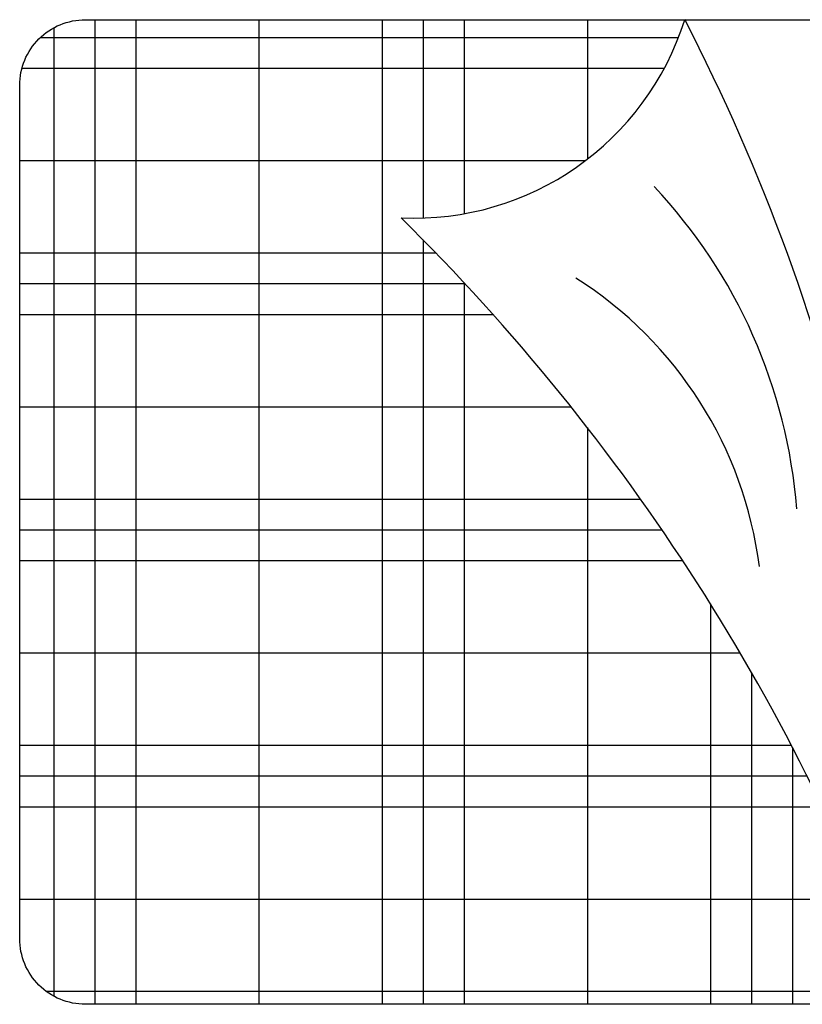
# Model space of a CAD drawing. Units: inches. Extents: x 3064 to 19385, y 846 to 15425.
# Tile 68 of 108: x 6533 to 6580, y 1625 to 1685. Entities that reach past the tile are written whole.
import ezdxf

# ---------------------------------------------------------------- set-up
doc = ezdxf.new("R2010")
doc.units = ezdxf.units.IN
doc.layers.add('A-FLOR-FIXT', color=9, linetype='Continuous', lineweight=18)
doc.layers.add('BLOCK', color=6, linetype='Continuous')

# ---------------------------------------------------------------- blocks, each defined once
blk = doc.blocks.new('*X5')
at = {"color": 0}
for p, q in [((276.598, 451.25), (280.51, 451.25)), ((275.455, 450.625), (280.51, 450.625)), ((274.411, 450), (280.51, 450)), ((265.51, 448.125), (267.634, 448.125)), ((271.723, 448.125), (280.51, 448.125)), ((265.51, 446.25), (268.465, 446.25)), ((269.519, 446.25), (280.51, 446.25)), ((265.51, 445.625), (268.531, 445.625)), ((268.866, 445.625), (280.51, 445.625)), ((265.51, 445), (280.51, 445)), ((265.51, 443.125), (280.51, 443.125)), ((265.51, 441.25), (280.51, 441.25)), ((265.51, 440.625), (280.51, 440.625)), ((265.634, 440), (280.386, 440))]:
    blk.add_line(p, q, dxfattribs=at)
blk = doc.blocks.new('*X6')
at = {"color": 0}
for p, q in [((280.312, 439.886), (280.312, 452.896)), ((278.906, 439.482), (278.906, 452.338)), ((277.5, 439.482), (277.5, 451.702)), ((277.031, 439.482), (277.031, 451.471)), ((276.562, 439.482), (276.562, 451.231)), ((275.156, 439.482), (275.156, 450.451)), ((273.75, 439.482), (273.75, 449.576)), ((265.781, 439.797), (265.781, 449.511)), ((266.25, 439.517), (266.25, 449.296)), ((273.281, 439.482), (273.281, 449.261)), ((272.812, 439.482), (272.812, 448.934)), ((267.656, 439.482), (267.656, 448.095)), ((271.406, 439.482), (271.406, 447.876)), ((270, 439.482), (270, 446.689)), ((269.531, 439.482), (269.531, 446.262)), ((269.062, 439.482), (269.062, 445.817))]:
    blk.add_line(p, q, dxfattribs=at)
blk = doc.blocks.new('A$C52E67D0D')
at = {"layer": 'BLOCK'}
blk.add_lwpolyline([(1901, 0), (601, 0, -0.414214), (501, 100), (501, 1700, -0.414214), (601, 1800), (1901, 1800, -0.414214), (2001, 1700), (2001, 100, -0.414214)], format="xyb", close=True, dxfattribs=at)
for centre, radius, start, end in [((1888.6, -1664.5), 3015.3, 87.8642, 117.4001), ((3101, -1685.8), 3227.7, 109.926, 135.3977), ((1308.8, 377.9), 807.6, 94.4436, 133.2788), ((1410.8, 520.2), 610.8, 97.2157, 147.6656), ((371.4, 600.4), 432, 357.3792, 72.5379)]:
    blk.add_arc(centre, radius, start, end, dxfattribs=at)
at = {"layer": 'BLOCK', "xscale": 100, "yscale": 100, "zscale": 100}
for name in ['*X6', '*X5']:
    blk.add_blockref(name, (-26050, -43948.2), dxfattribs=at)

msp = doc.modelspace()

# ---------------------------------------------------------------- block references
at = {"layer": 'A-FLOR-FIXT', "xscale": 0.039370099999992, "yscale": 0.039370099999992, "zscale": 0.039370099999992, "rotation": 270}
msp.add_blockref('A$C52E67D0D', (6533.167, 1704.241), dxfattribs=at)

doc.saveas('drawing.dxf')
